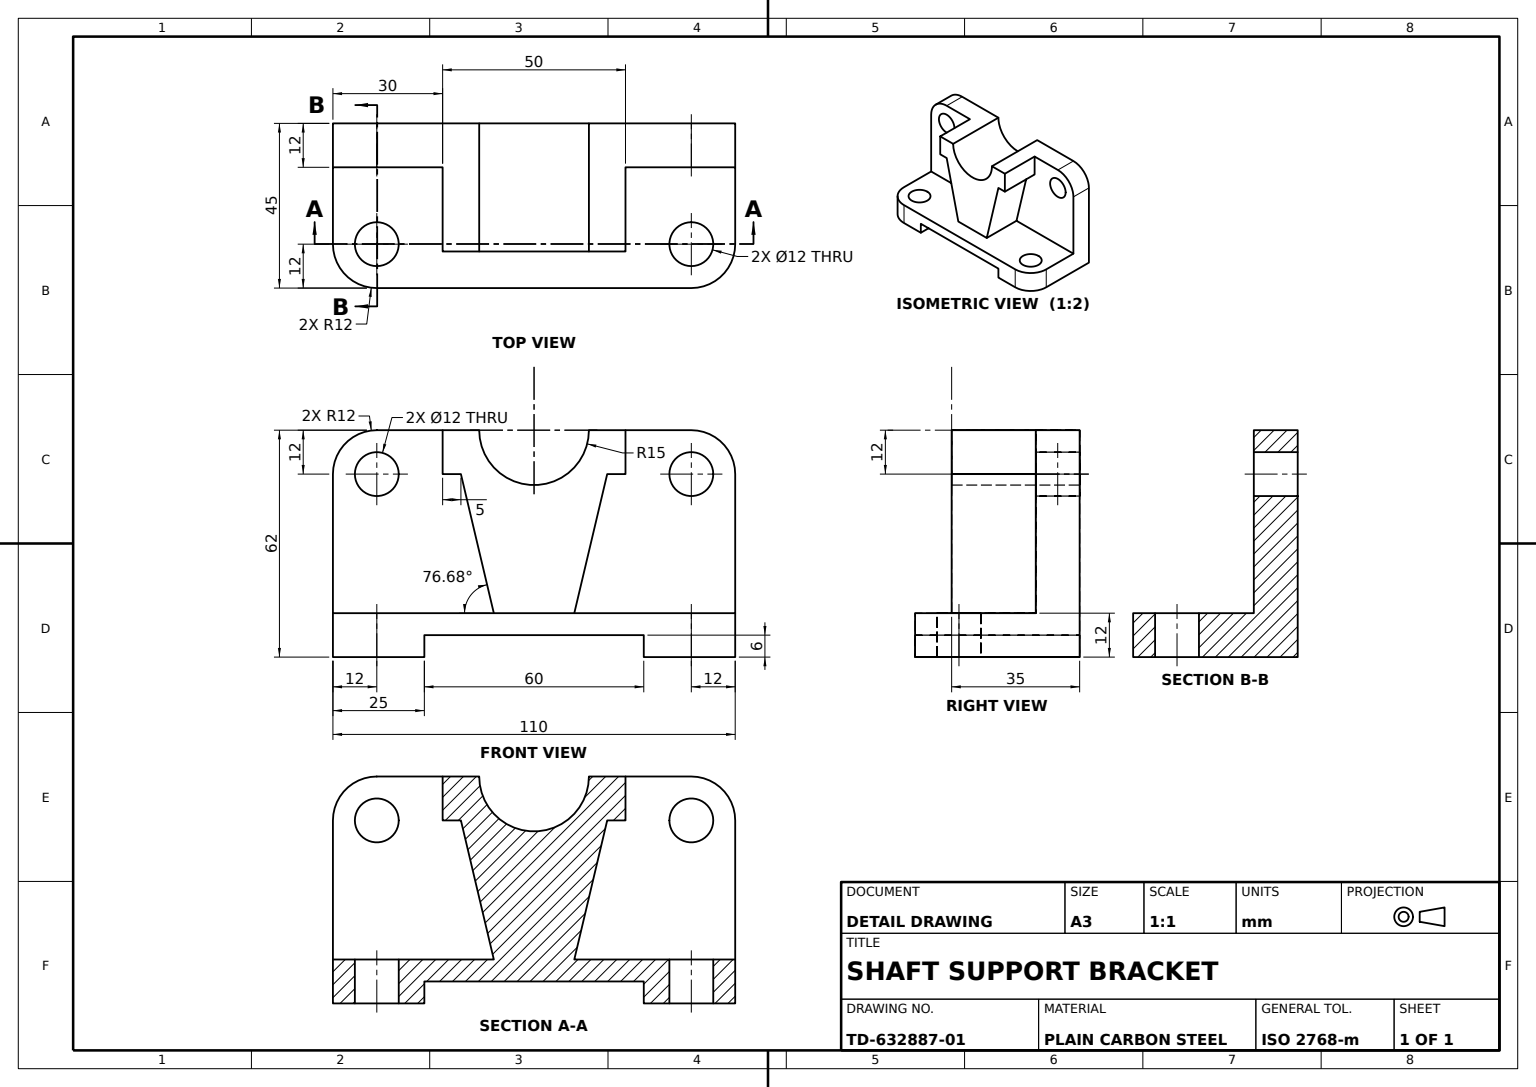
from build123d import *

# Parameters (mm, degrees)
BASE_PLATE_SKETCH_R            = 6
BASE_PLATE_110X45X12_DEPTH     = 12
BACK_WALL_SKETCH_R             = 6
BACK_WALL_12MM_DEPTH           = 12
BASE_UNDERSIDE_SLOT_SKETCH_W   = 60
BASE_UNDERSIDE_SLOT_SKETCH_H   = 6
BASE_UNDERSIDE_SLOT_60X6_DEPTH = 80
TROUGH_BORE_SKETCH_R           = 15
TROUGH_BORE_CUT_DEPTH          = 80
PEDESTAL_BLOCK_DEPTH           = 35
PEDESTAL_START                 = -23
PEDESTAL_SIDE_TRIM_CUT_DEPTH   = 23
PEDESTAL_START_2               = -35
PEDESTAL_WEB_BOSS_DEPTH        = 35


with BuildPart() as part:
    # Base Plate Sketch → Base Plate 110x45x12 (new body)
    with BuildSketch(Plane(origin=(0, 0, 0), x_dir=(1, 0, 0), z_dir=(0, 1, 0))):
        with BuildLine():
            Line((-55, 22.5), (55, 22.5))
            Line((55, 22.5), (55, -10.5))
            ThreePointArc((55, -10.5), (51.485281374, -18.985281374), (43, -22.5))
            Line((43, -22.5), (-43, -22.5))
            ThreePointArc((-43, -22.5), (-51.485281374, -18.985281374), (-55, -10.5))
            Line((-55, -10.5), (-55, 22.5))
        make_face()
        with Locations(Location((-43, -10.5, 0), (0, 0, 270))):
            Circle(BASE_PLATE_SKETCH_R, mode=Mode.SUBTRACT)
        with Locations(Location((43, -10.5, 0), (0, 0, 270))):
            Circle(BASE_PLATE_SKETCH_R, mode=Mode.SUBTRACT)
    extrude(amount=BASE_PLATE_110X45X12_DEPTH)

    # Back Wall Sketch → Back Wall 12mm (add)
    with BuildSketch(Plane(origin=(0, 0, -22.5), x_dir=(-1, 0, 0), z_dir=(0, 0, -1))):
        with BuildLine():
            Line((-55, 0), (55, 0))
            Line((55, 0), (55, 50))
            ThreePointArc((55, 50), (51.485281374, 58.485281374), (43, 62))
            Line((43, 62), (-43, 62))
            ThreePointArc((-43, 62), (-51.485281374, 58.485281374), (-55, 50))
            Line((-55, 50), (-55, 0))
        make_face()
        with Locations((-43, 50)):
            Circle(BACK_WALL_SKETCH_R, mode=Mode.SUBTRACT)
        with Locations((43, 50)):
            Circle(BACK_WALL_SKETCH_R, mode=Mode.SUBTRACT)
    extrude(amount=-BACK_WALL_12MM_DEPTH)

    # Base Underside Slot Sketch → Base Underside Slot 60x6 (cut)
    with BuildSketch(Plane.XY.offset(22.5)):
        with Locations((0, 3)):
            Rectangle(BASE_UNDERSIDE_SLOT_SKETCH_W, BASE_UNDERSIDE_SLOT_SKETCH_H)
    extrude(amount=-BASE_UNDERSIDE_SLOT_60X6_DEPTH, mode=Mode.SUBTRACT)

    # Trough Bore Sketch → Trough Bore Cut (cut)
    with BuildSketch(Plane(origin=(0, 0, -22.5), x_dir=(-1, 0, 0), z_dir=(0, 0, -1))):
        with Locations((0, 62)):
            Circle(TROUGH_BORE_SKETCH_R)
    extrude(amount=-TROUGH_BORE_CUT_DEPTH, mode=Mode.SUBTRACT)

    # Pedestal Block Sketch → Pedestal Block (add)
    with BuildSketch(Plane(origin=(0, 0, -22.5), x_dir=(-1, 0, 0), z_dir=(0, 0, -1))):
        with BuildLine():
            Line((-25, 62), (-15, 62))
            ThreePointArc((-15, 62), (0, 47), (15, 62))
            Line((15, 62), (25, 62))
            ThreePointArc((25, 62), (0, 37), (-25, 62))
        make_face()
    extrude(amount=-PEDESTAL_BLOCK_DEPTH)

    # Pedestal Profile Sketch → Pedestal Side Trim Cut (cut)
    with BuildSketch(Plane.XY.offset(12.5).offset(PEDESTAL_START)):
        with BuildLine():
            ThreePointArc((-21.931712199, 50), (-20.572082469, 47.794739605), (-18.991532718, 45.742027032))
            Line((-18.991532718, 45.742027032), (-20, 50))
            Line((-20, 50), (-21.931712199, 50))
        make_face()
        with BuildLine():
            Line((20, 50), (18.991532718, 45.742027032))
            ThreePointArc((18.991532718, 45.742027032), (20.572082469, 47.794739605), (21.931712199, 50))
            Line((21.931712199, 50), (20, 50))
        make_face()
    extrude(amount=PEDESTAL_SIDE_TRIM_CUT_DEPTH, mode=Mode.SUBTRACT)

    # Sketch6_3 → Pedestal Web Boss (add)
    with BuildSketch(Plane.XY.offset(12.5).offset(PEDESTAL_START_2)):
        with BuildLine():
            Line((-20, 50), (-18.991532718, 45.742027032))
            ThreePointArc((-18.991532718, 45.742027032), (0, 37), (18.991532718, 45.742027032))
            Line((18.991532718, 45.742027032), (20, 50))
            Line((20, 50), (21.931712199, 50))
            ThreePointArc((21.931712199, 50), (24.220784514, 55.806971863), (25, 62))
            Line((25, 62), (15, 62))
            ThreePointArc((15, 62), (0, 47), (-15, 62))
            Line((-15, 62), (-25, 62))
            ThreePointArc((-25, 62), (-24.220784514, 55.806971863), (-21.931712199, 50))
            Line((-21.931712199, 50), (-20, 50))
        make_face()
        with BuildLine():
            Line((-25, 50), (-21.931712199, 50))
            ThreePointArc((-21.931712199, 50), (-24.220784514, 55.806971863), (-25, 62))
            Line((-25, 62), (-25, 50))
        make_face()
        with BuildLine():
            ThreePointArc((25, 62), (24.220784514, 55.806971863), (21.931712199, 50))
            Line((21.931712199, 50), (25, 50))
            Line((25, 50), (25, 62))
        make_face()
        with BuildLine():
            Line((-18.991532718, 45.742027032), (-11, 12))
            Line((-11, 12), (11, 12))
            Line((11, 12), (18.991532718, 45.742027032))
            ThreePointArc((18.991532718, 45.742027032), (0, 37), (-18.991532718, 45.742027032))
        make_face()
    extrude(amount=PEDESTAL_WEB_BOSS_DEPTH)


solid = part.part
